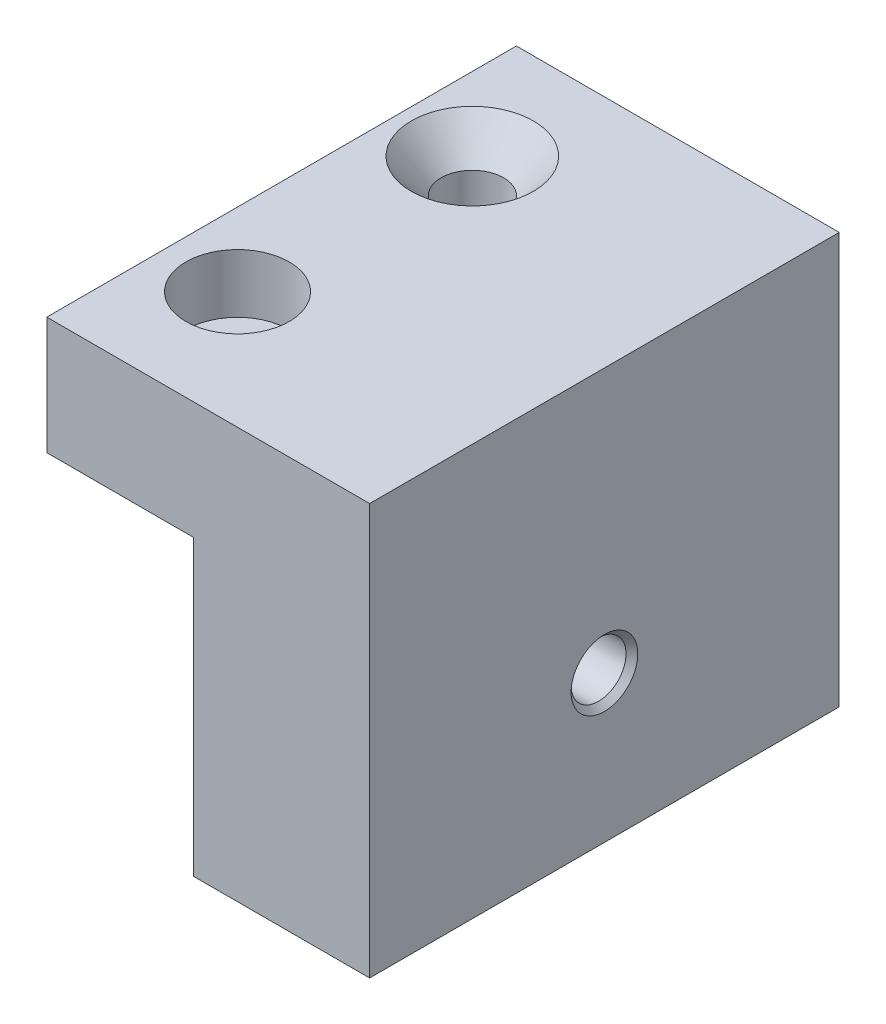
ISO-10303-21;
HEADER;
FILE_DESCRIPTION(('STEP AP214'),'2;1');
FILE_NAME('part.step','',(''),(''),'','','');
FILE_SCHEMA(('AUTOMOTIVE_DESIGN { 1 0 10303 214 1 1 1 1 }'));
ENDSEC;
DATA;
#1=APPLICATION_CONTEXT('core data for automotive mechanical design processes');
#2=APPLICATION_PROTOCOL_DEFINITION('international standard','automotive_design',2000,#1);
#3=PRODUCT_CONTEXT('',#1,'mechanical');
#4=PRODUCT('Part','Part','',(#3));
#5=PRODUCT_RELATED_PRODUCT_CATEGORY('part','',(#4));
#6=PRODUCT_DEFINITION_FORMATION('','',#4);
#7=PRODUCT_DEFINITION_CONTEXT('part definition',#1,'design');
#8=PRODUCT_DEFINITION('design','',#6,#7);
#9=PRODUCT_DEFINITION_SHAPE('','',#8);
#10=(LENGTH_UNIT() NAMED_UNIT(*) SI_UNIT(.MILLI.,.METRE.));
#11=(NAMED_UNIT(*) PLANE_ANGLE_UNIT() SI_UNIT($,.RADIAN.));
#12=(NAMED_UNIT(*) SI_UNIT($,.STERADIAN.) SOLID_ANGLE_UNIT());
#13=UNCERTAINTY_MEASURE_WITH_UNIT(LENGTH_MEASURE(1.E-05),#10,'distance_accuracy_value','');
#14=(GEOMETRIC_REPRESENTATION_CONTEXT(3) GLOBAL_UNCERTAINTY_ASSIGNED_CONTEXT((#13)) GLOBAL_UNIT_ASSIGNED_CONTEXT((#10,
#11,#12)) REPRESENTATION_CONTEXT('',''));
#15=CARTESIAN_POINT('',(0.,0.,0.));
#16=DIRECTION('',(0.,0.,1.));
#17=DIRECTION('',(1.,0.,0.));
#18=AXIS2_PLACEMENT_3D('',#15,#16,#17);
#19=CARTESIAN_POINT('',(-15.875,0.,50.8));
#20=DIRECTION('',(1.,0.,0.));
#21=DIRECTION('',(0.,0.,-1.));
#22=AXIS2_PLACEMENT_3D('',#19,#20,#21);
#23=PLANE('',#22);
#24=DIRECTION('',(0.,-1.,0.));
#25=VECTOR('',#24,1.);
#26=CARTESIAN_POINT('',(-15.875,0.,0.));
#27=LINE('',#26,#25);
#28=CARTESIAN_POINT('',(-15.875,12.7,0.));
#29=VERTEX_POINT('',#28);
#30=CARTESIAN_POINT('',(-15.875,0.,0.));
#31=VERTEX_POINT('',#30);
#32=EDGE_CURVE('E137',#29,#31,#27,.T.);
#33=ORIENTED_EDGE('',*,*,#32,.T.);
#34=DIRECTION('',(0.,0.,-1.));
#35=VECTOR('',#34,1.);
#36=CARTESIAN_POINT('',(-15.875,0.,50.8));
#37=LINE('',#36,#35);
#38=CARTESIAN_POINT('',(-15.875,0.,50.8));
#39=VERTEX_POINT('',#38);
#40=EDGE_CURVE('E146',#39,#31,#37,.T.);
#41=ORIENTED_EDGE('',*,*,#40,.F.);
#42=DIRECTION('',(0.,-1.,0.));
#43=VECTOR('',#42,1.);
#44=CARTESIAN_POINT('',(-15.875,0.,50.8));
#45=LINE('',#44,#43);
#46=CARTESIAN_POINT('',(-15.875,12.7,50.8));
#47=VERTEX_POINT('',#46);
#48=EDGE_CURVE('E103',#47,#39,#45,.T.);
#49=ORIENTED_EDGE('',*,*,#48,.F.);
#50=DIRECTION('',(0.,0.,-1.));
#51=VECTOR('',#50,1.);
#52=CARTESIAN_POINT('',(-15.875,12.7,50.8));
#53=LINE('',#52,#51);
#54=EDGE_CURVE('E155',#47,#29,#53,.T.);
#55=ORIENTED_EDGE('',*,*,#54,.T.);
#56=EDGE_LOOP('',(#33,#41,#49,#55));
#57=FACE_BOUND('',#56,.T.);
#58=ADVANCED_FACE('F41',(#57),#23,.F.);
#59=CARTESIAN_POINT('',(0.,0.,50.8));
#60=DIRECTION('',(0.,1.,0.));
#61=DIRECTION('',(-1.,0.,0.));
#62=AXIS2_PLACEMENT_3D('',#59,#60,#61);
#63=PLANE('',#62);
#64=CARTESIAN_POINT('',(-7.93749999999999,0.,38.1));
#65=DIRECTION('',(0.,1.,0.));
#66=DIRECTION('',(-1.,0.,0.));
#67=AXIS2_PLACEMENT_3D('',#64,#65,#66);
#68=CIRCLE('',#67,3.37819999999999);
#69=CARTESIAN_POINT('',(-11.3157,0.,38.1));
#70=VERTEX_POINT('',#69);
#71=EDGE_CURVE('E46',#70,#70,#68,.T.);
#72=ORIENTED_EDGE('',*,*,#71,.T.);
#73=EDGE_LOOP('',(#72));
#74=FACE_BOUND('',#73,.T.);
#75=CARTESIAN_POINT('',(-7.93749999999999,0.,12.7));
#76=DIRECTION('',(0.,1.,0.));
#77=DIRECTION('',(-1.,0.,0.));
#78=AXIS2_PLACEMENT_3D('',#75,#76,#77);
#79=CIRCLE('',#78,3.3782);
#80=CARTESIAN_POINT('',(-11.3157,0.,12.7));
#81=VERTEX_POINT('',#80);
#82=EDGE_CURVE('E163',#81,#81,#79,.T.);
#83=ORIENTED_EDGE('',*,*,#82,.T.);
#84=EDGE_LOOP('',(#83));
#85=FACE_BOUND('',#84,.T.);
#86=CARTESIAN_POINT('',(-7.9375,0.,25.4));
#87=DIRECTION('',(0.,-1.,0.));
#88=DIRECTION('',(0.,0.,-1.));
#89=AXIS2_PLACEMENT_3D('',#86,#87,#88);
#90=CIRCLE('',#89,1.6002);
#91=CARTESIAN_POINT('',(-7.9375,0.,23.7998));
#92=VERTEX_POINT('',#91);
#93=EDGE_CURVE('E161',#92,#92,#90,.T.);
#94=ORIENTED_EDGE('',*,*,#93,.F.);
#95=EDGE_LOOP('',(#94));
#96=FACE_BOUND('',#95,.T.);
#97=DIRECTION('',(1.,0.,0.));
#98=VECTOR('',#97,1.);
#99=CARTESIAN_POINT('',(0.,0.,0.));
#100=LINE('',#99,#98);
#101=CARTESIAN_POINT('',(0.,0.,0.));
#102=VERTEX_POINT('',#101);
#103=EDGE_CURVE('E139',#31,#102,#100,.T.);
#104=ORIENTED_EDGE('',*,*,#103,.T.);
#105=DIRECTION('',(0.,0.,-1.));
#106=VECTOR('',#105,1.);
#107=CARTESIAN_POINT('',(0.,0.,50.8));
#108=LINE('',#107,#106);
#109=CARTESIAN_POINT('',(0.,0.,50.8));
#110=VERTEX_POINT('',#109);
#111=EDGE_CURVE('E123',#110,#102,#108,.T.);
#112=ORIENTED_EDGE('',*,*,#111,.F.);
#113=DIRECTION('',(1.,0.,0.));
#114=VECTOR('',#113,1.);
#115=CARTESIAN_POINT('',(0.,0.,50.8));
#116=LINE('',#115,#114);
#117=EDGE_CURVE('E116',#39,#110,#116,.T.);
#118=ORIENTED_EDGE('',*,*,#117,.F.);
#119=ORIENTED_EDGE('',*,*,#40,.T.);
#120=EDGE_LOOP('',(#104,#112,#118,#119));
#121=FACE_BOUND('',#120,.T.);
#122=ADVANCED_FACE('F183',(#74,#85,#96,#121),#63,.F.);
#123=CARTESIAN_POINT('',(0.,0.,50.8));
#124=DIRECTION('',(1.,0.,0.));
#125=DIRECTION('',(0.,1.,0.));
#126=AXIS2_PLACEMENT_3D('',#123,#124,#125);
#127=PLANE('',#126);
#128=CARTESIAN_POINT('',(0.,-15.875,25.4));
#129=DIRECTION('',(1.,0.,0.));
#130=DIRECTION('',(0.,1.,0.));
#131=AXIS2_PLACEMENT_3D('',#128,#129,#130);
#132=CIRCLE('',#131,3.6068);
#133=CARTESIAN_POINT('',(0.,-12.2682,25.4));
#134=VERTEX_POINT('',#133);
#135=EDGE_CURVE('E11',#134,#134,#132,.T.);
#136=ORIENTED_EDGE('',*,*,#135,.T.);
#137=EDGE_LOOP('',(#136));
#138=FACE_BOUND('',#137,.T.);
#139=DIRECTION('',(0.,-1.,0.));
#140=VECTOR('',#139,1.);
#141=CARTESIAN_POINT('',(0.,0.,0.));
#142=LINE('',#141,#140);
#143=CARTESIAN_POINT('',(0.,-31.75,0.));
#144=VERTEX_POINT('',#143);
#145=EDGE_CURVE('E121',#102,#144,#142,.T.);
#146=ORIENTED_EDGE('',*,*,#145,.T.);
#147=DIRECTION('',(0.,0.,-1.));
#148=VECTOR('',#147,1.);
#149=CARTESIAN_POINT('',(0.,-31.75,50.8));
#150=LINE('',#149,#148);
#151=CARTESIAN_POINT('',(0.,-31.75,50.8));
#152=VERTEX_POINT('',#151);
#153=EDGE_CURVE('E122',#152,#144,#150,.T.);
#154=ORIENTED_EDGE('',*,*,#153,.F.);
#155=DIRECTION('',(0.,-1.,0.));
#156=VECTOR('',#155,1.);
#157=CARTESIAN_POINT('',(0.,0.,50.8));
#158=LINE('',#157,#156);
#159=EDGE_CURVE('E109',#110,#152,#158,.T.);
#160=ORIENTED_EDGE('',*,*,#159,.F.);
#161=ORIENTED_EDGE('',*,*,#111,.T.);
#162=EDGE_LOOP('',(#146,#154,#160,#161));
#163=FACE_BOUND('',#162,.T.);
#164=ADVANCED_FACE('F125',(#138,#163),#127,.F.);
#165=CARTESIAN_POINT('',(0.,-31.75,50.8));
#166=DIRECTION('',(0.,1.,0.));
#167=DIRECTION('',(0.,0.,1.));
#168=AXIS2_PLACEMENT_3D('',#165,#166,#167);
#169=PLANE('',#168);
#170=DIRECTION('',(1.,0.,0.));
#171=VECTOR('',#170,1.);
#172=CARTESIAN_POINT('',(0.,-31.75,0.));
#173=LINE('',#172,#171);
#174=CARTESIAN_POINT('',(19.05,-31.75,0.));
#175=VERTEX_POINT('',#174);
#176=EDGE_CURVE('E86',#144,#175,#173,.T.);
#177=ORIENTED_EDGE('',*,*,#176,.T.);
#178=DIRECTION('',(0.,0.,-1.));
#179=VECTOR('',#178,1.);
#180=CARTESIAN_POINT('',(19.05,-31.75,50.8));
#181=LINE('',#180,#179);
#182=CARTESIAN_POINT('',(19.05,-31.75,50.8));
#183=VERTEX_POINT('',#182);
#184=EDGE_CURVE('E127',#183,#175,#181,.T.);
#185=ORIENTED_EDGE('',*,*,#184,.F.);
#186=DIRECTION('',(1.,0.,0.));
#187=VECTOR('',#186,1.);
#188=CARTESIAN_POINT('',(0.,-31.75,50.8));
#189=LINE('',#188,#187);
#190=EDGE_CURVE('E112',#152,#183,#189,.T.);
#191=ORIENTED_EDGE('',*,*,#190,.F.);
#192=ORIENTED_EDGE('',*,*,#153,.T.);
#193=EDGE_LOOP('',(#177,#185,#191,#192));
#194=FACE_BOUND('',#193,.T.);
#195=ADVANCED_FACE('F129',(#194),#169,.F.);
#196=CARTESIAN_POINT('',(19.05,12.7,50.8));
#197=DIRECTION('',(-1.,0.,0.));
#198=DIRECTION('',(0.,-1.,0.));
#199=AXIS2_PLACEMENT_3D('',#196,#197,#198);
#200=PLANE('',#199);
#201=CARTESIAN_POINT('',(19.05,-15.875,25.4));
#202=DIRECTION('',(-1.,0.,0.));
#203=DIRECTION('',(0.,-1.,0.));
#204=AXIS2_PLACEMENT_3D('',#201,#202,#203);
#205=CIRCLE('',#204,3.6068);
#206=CARTESIAN_POINT('',(19.05,-19.4818,25.4));
#207=VERTEX_POINT('',#206);
#208=EDGE_CURVE('E153',#207,#207,#205,.T.);
#209=ORIENTED_EDGE('',*,*,#208,.T.);
#210=EDGE_LOOP('',(#209));
#211=FACE_BOUND('',#210,.T.);
#212=DIRECTION('',(0.,1.,0.));
#213=VECTOR('',#212,1.);
#214=CARTESIAN_POINT('',(19.05,12.7,0.));
#215=LINE('',#214,#213);
#216=CARTESIAN_POINT('',(19.05,12.7,0.));
#217=VERTEX_POINT('',#216);
#218=EDGE_CURVE('E94',#175,#217,#215,.T.);
#219=ORIENTED_EDGE('',*,*,#218,.T.);
#220=DIRECTION('',(0.,0.,-1.));
#221=VECTOR('',#220,1.);
#222=CARTESIAN_POINT('',(19.05,12.7,50.8));
#223=LINE('',#222,#221);
#224=CARTESIAN_POINT('',(19.05,12.7,50.8));
#225=VERTEX_POINT('',#224);
#226=EDGE_CURVE('E135',#225,#217,#223,.T.);
#227=ORIENTED_EDGE('',*,*,#226,.F.);
#228=DIRECTION('',(0.,1.,0.));
#229=VECTOR('',#228,1.);
#230=CARTESIAN_POINT('',(19.05,12.7,50.8));
#231=LINE('',#230,#229);
#232=EDGE_CURVE('E128',#183,#225,#231,.T.);
#233=ORIENTED_EDGE('',*,*,#232,.F.);
#234=ORIENTED_EDGE('',*,*,#184,.T.);
#235=EDGE_LOOP('',(#219,#227,#233,#234));
#236=FACE_BOUND('',#235,.T.);
#237=ADVANCED_FACE('F186',(#211,#236),#200,.F.);
#238=CARTESIAN_POINT('',(0.,12.7,50.8));
#239=DIRECTION('',(0.,-1.,0.));
#240=DIRECTION('',(0.,0.,-1.));
#241=AXIS2_PLACEMENT_3D('',#238,#239,#240);
#242=PLANE('',#241);
#243=CARTESIAN_POINT('',(-7.93749999999999,12.7,38.1));
#244=DIRECTION('',(0.,1.,0.));
#245=DIRECTION('',(0.,0.,1.));
#246=AXIS2_PLACEMENT_3D('',#243,#244,#245);
#247=CIRCLE('',#246,5.588);
#248=CARTESIAN_POINT('',(-7.93749999999999,12.7,43.688));
#249=VERTEX_POINT('',#248);
#250=EDGE_CURVE('E380',#249,#249,#247,.T.);
#251=ORIENTED_EDGE('',*,*,#250,.F.);
#252=EDGE_LOOP('',(#251));
#253=FACE_BOUND('',#252,.T.);
#254=CARTESIAN_POINT('',(-7.93749999999999,12.7,12.7));
#255=DIRECTION('',(0.,1.,0.));
#256=DIRECTION('',(0.,0.,1.));
#257=AXIS2_PLACEMENT_3D('',#254,#255,#256);
#258=CIRCLE('',#257,6.604);
#259=CARTESIAN_POINT('',(-7.93749999999999,12.7,19.304));
#260=VERTEX_POINT('',#259);
#261=EDGE_CURVE('E167',#260,#260,#258,.T.);
#262=ORIENTED_EDGE('',*,*,#261,.F.);
#263=EDGE_LOOP('',(#262));
#264=FACE_BOUND('',#263,.T.);
#265=DIRECTION('',(-1.,0.,0.));
#266=VECTOR('',#265,1.);
#267=CARTESIAN_POINT('',(0.,12.7,0.));
#268=LINE('',#267,#266);
#269=EDGE_CURVE('E144',#217,#29,#268,.T.);
#270=ORIENTED_EDGE('',*,*,#269,.T.);
#271=ORIENTED_EDGE('',*,*,#54,.F.);
#272=DIRECTION('',(-1.,0.,0.));
#273=VECTOR('',#272,1.);
#274=CARTESIAN_POINT('',(0.,12.7,50.8));
#275=LINE('',#274,#273);
#276=EDGE_CURVE('E62',#225,#47,#275,.T.);
#277=ORIENTED_EDGE('',*,*,#276,.F.);
#278=ORIENTED_EDGE('',*,*,#226,.T.);
#279=EDGE_LOOP('',(#270,#271,#277,#278));
#280=FACE_BOUND('',#279,.T.);
#281=ADVANCED_FACE('F189',(#253,#264,#280),#242,.F.);
#282=CARTESIAN_POINT('',(0.,0.,50.8));
#283=DIRECTION('',(0.,0.,-1.));
#284=DIRECTION('',(-1.,0.,0.));
#285=AXIS2_PLACEMENT_3D('',#282,#283,#284);
#286=PLANE('',#285);
#287=ORIENTED_EDGE('',*,*,#276,.T.);
#288=ORIENTED_EDGE('',*,*,#48,.T.);
#289=ORIENTED_EDGE('',*,*,#117,.T.);
#290=ORIENTED_EDGE('',*,*,#159,.T.);
#291=ORIENTED_EDGE('',*,*,#190,.T.);
#292=ORIENTED_EDGE('',*,*,#232,.T.);
#293=EDGE_LOOP('',(#287,#288,#289,#290,#291,#292));
#294=FACE_BOUND('',#293,.T.);
#295=ADVANCED_FACE('F115',(#294),#286,.F.);
#296=CARTESIAN_POINT('',(0.,0.,0.));
#297=DIRECTION('',(0.,0.,-1.));
#298=DIRECTION('',(-1.,0.,0.));
#299=AXIS2_PLACEMENT_3D('',#296,#297,#298);
#300=PLANE('',#299);
#301=ORIENTED_EDGE('',*,*,#32,.F.);
#302=ORIENTED_EDGE('',*,*,#269,.F.);
#303=ORIENTED_EDGE('',*,*,#218,.F.);
#304=ORIENTED_EDGE('',*,*,#176,.F.);
#305=ORIENTED_EDGE('',*,*,#145,.F.);
#306=ORIENTED_EDGE('',*,*,#103,.F.);
#307=EDGE_LOOP('',(#301,#302,#303,#304,#305,#306));
#308=FACE_BOUND('',#307,.T.);
#309=ADVANCED_FACE('F187',(#308),#300,.T.);
#310=CARTESIAN_POINT('',(0.,-15.875,25.4));
#311=DIRECTION('',(-1.,0.,0.));
#312=DIRECTION('',(0.,0.,1.));
#313=AXIS2_PLACEMENT_3D('',#310,#311,#312);
#314=CYLINDRICAL_SURFACE('',#313,2.97179999999999);
#315=CARTESIAN_POINT('',(18.415,-15.875,25.4));
#316=DIRECTION('',(-1.,0.,0.));
#317=DIRECTION('',(0.,0.,1.));
#318=AXIS2_PLACEMENT_3D('',#315,#316,#317);
#319=CIRCLE('',#318,2.97179999999999);
#320=CARTESIAN_POINT('',(18.415,-15.875,28.3718));
#321=VERTEX_POINT('',#320);
#322=EDGE_CURVE('E55',#321,#321,#319,.F.);
#323=ORIENTED_EDGE('',*,*,#322,.T.);
#324=EDGE_LOOP('',(#323));
#325=FACE_BOUND('',#324,.T.);
#326=CARTESIAN_POINT('',(0.635,-15.875,25.4));
#327=DIRECTION('',(1.,0.,0.));
#328=DIRECTION('',(0.,0.,-1.));
#329=AXIS2_PLACEMENT_3D('',#326,#327,#328);
#330=CIRCLE('',#329,2.97179999999999);
#331=CARTESIAN_POINT('',(0.635,-15.875,22.4282));
#332=VERTEX_POINT('',#331);
#333=EDGE_CURVE('E160',#332,#332,#330,.F.);
#334=ORIENTED_EDGE('',*,*,#333,.T.);
#335=EDGE_LOOP('',(#334));
#336=FACE_BOUND('',#335,.T.);
#337=ADVANCED_FACE('F213',(#325,#336),#314,.F.);
#338=CARTESIAN_POINT('',(19.05,-15.875,25.4));
#339=DIRECTION('',(1.,0.,0.));
#340=DIRECTION('',(0.,0.,-1.));
#341=AXIS2_PLACEMENT_3D('',#338,#339,#340);
#342=CONICAL_SURFACE('',#341,3.6068,0.785398163397441);
#343=ORIENTED_EDGE('',*,*,#322,.F.);
#344=EDGE_LOOP('',(#343));
#345=FACE_BOUND('',#344,.T.);
#346=ORIENTED_EDGE('',*,*,#208,.F.);
#347=EDGE_LOOP('',(#346));
#348=FACE_BOUND('',#347,.T.);
#349=ADVANCED_FACE('F212',(#345,#348),#342,.F.);
#350=CARTESIAN_POINT('',(0.635,-15.875,25.4));
#351=DIRECTION('',(-1.,0.,0.));
#352=DIRECTION('',(0.,0.,1.));
#353=AXIS2_PLACEMENT_3D('',#350,#351,#352);
#354=CONICAL_SURFACE('',#353,2.97179999999999,0.785398163397453);
#355=ORIENTED_EDGE('',*,*,#135,.F.);
#356=EDGE_LOOP('',(#355));
#357=FACE_BOUND('',#356,.T.);
#358=ORIENTED_EDGE('',*,*,#333,.F.);
#359=EDGE_LOOP('',(#358));
#360=FACE_BOUND('',#359,.T.);
#361=ADVANCED_FACE('F42',(#357,#360),#354,.F.);
#362=CARTESIAN_POINT('',(-7.9375,6.0198,25.4));
#363=DIRECTION('',(0.,-1.,0.));
#364=DIRECTION('',(0.,0.,-1.));
#365=AXIS2_PLACEMENT_3D('',#362,#363,#364);
#366=CONICAL_SURFACE('',#365,1.6002,0.785398163397447);
#367=CARTESIAN_POINT('',(-7.9375,7.62,25.4));
#368=VERTEX_POINT('',#367);
#369=VERTEX_LOOP('',#368);
#370=FACE_BOUND('',#369,.T.);
#371=CARTESIAN_POINT('',(-7.9375,6.0198,25.4));
#372=DIRECTION('',(0.,-1.,0.));
#373=DIRECTION('',(0.,0.,-1.));
#374=AXIS2_PLACEMENT_3D('',#371,#372,#373);
#375=CIRCLE('',#374,1.6002);
#376=CARTESIAN_POINT('',(-7.9375,6.0198,23.7998));
#377=VERTEX_POINT('',#376);
#378=EDGE_CURVE('E136',#377,#377,#375,.T.);
#379=ORIENTED_EDGE('',*,*,#378,.T.);
#380=EDGE_LOOP('',(#379));
#381=FACE_BOUND('',#380,.T.);
#382=ADVANCED_FACE('F219',(#370,#381),#366,.F.);
#383=CARTESIAN_POINT('',(-7.9375,0.,25.4));
#384=DIRECTION('',(0.,-1.,0.));
#385=DIRECTION('',(0.,0.,-1.));
#386=AXIS2_PLACEMENT_3D('',#383,#384,#385);
#387=CYLINDRICAL_SURFACE('',#386,1.6002);
#388=ORIENTED_EDGE('',*,*,#378,.F.);
#389=EDGE_LOOP('',(#388));
#390=FACE_BOUND('',#389,.T.);
#391=ORIENTED_EDGE('',*,*,#93,.T.);
#392=EDGE_LOOP('',(#391));
#393=FACE_BOUND('',#392,.T.);
#394=ADVANCED_FACE('F321',(#390,#393),#387,.F.);
#395=CARTESIAN_POINT('',(-7.93749999999999,12.7,12.7));
#396=DIRECTION('',(0.,1.,0.));
#397=DIRECTION('',(0.,0.,1.));
#398=AXIS2_PLACEMENT_3D('',#395,#396,#397);
#399=CYLINDRICAL_SURFACE('',#398,3.3782);
#400=CARTESIAN_POINT('',(-7.93749999999999,8.98914159198646,12.7));
#401=DIRECTION('',(0.,1.,0.));
#402=DIRECTION('',(0.,0.,1.));
#403=AXIS2_PLACEMENT_3D('',#400,#401,#402);
#404=CIRCLE('',#403,3.3782);
#405=CARTESIAN_POINT('',(-7.93749999999999,8.98914159198646,16.0782));
#406=VERTEX_POINT('',#405);
#407=EDGE_CURVE('E165',#406,#406,#404,.T.);
#408=ORIENTED_EDGE('',*,*,#407,.T.);
#409=EDGE_LOOP('',(#408));
#410=FACE_BOUND('',#409,.T.);
#411=ORIENTED_EDGE('',*,*,#82,.F.);
#412=EDGE_LOOP('',(#411));
#413=FACE_BOUND('',#412,.T.);
#414=ADVANCED_FACE('F314',(#410,#413),#399,.F.);
#415=CARTESIAN_POINT('',(-7.93749999999999,12.7,12.7));
#416=DIRECTION('',(0.,1.,0.));
#417=DIRECTION('',(0.,0.,1.));
#418=AXIS2_PLACEMENT_3D('',#415,#416,#417);
#419=CONICAL_SURFACE('',#418,6.604,0.715584993317675);
#420=ORIENTED_EDGE('',*,*,#407,.F.);
#421=EDGE_LOOP('',(#420));
#422=FACE_BOUND('',#421,.T.);
#423=ORIENTED_EDGE('',*,*,#261,.T.);
#424=EDGE_LOOP('',(#423));
#425=FACE_BOUND('',#424,.T.);
#426=ADVANCED_FACE('F287',(#422,#425),#419,.F.);
#427=CARTESIAN_POINT('',(-7.93749999999999,12.7,38.1));
#428=DIRECTION('',(0.,1.,0.));
#429=DIRECTION('',(0.,0.,1.));
#430=AXIS2_PLACEMENT_3D('',#427,#428,#429);
#431=CYLINDRICAL_SURFACE('',#430,3.37819999999999);
#432=CARTESIAN_POINT('',(-7.93749999999999,6.35,38.1));
#433=DIRECTION('',(0.,1.,0.));
#434=DIRECTION('',(0.,0.,1.));
#435=AXIS2_PLACEMENT_3D('',#432,#433,#434);
#436=CIRCLE('',#435,3.3782);
#437=CARTESIAN_POINT('',(-7.93749999999999,6.35,41.4782));
#438=VERTEX_POINT('',#437);
#439=EDGE_CURVE('E378',#438,#438,#436,.T.);
#440=ORIENTED_EDGE('',*,*,#439,.T.);
#441=EDGE_LOOP('',(#440));
#442=FACE_BOUND('',#441,.T.);
#443=ORIENTED_EDGE('',*,*,#71,.F.);
#444=EDGE_LOOP('',(#443));
#445=FACE_BOUND('',#444,.T.);
#446=ADVANCED_FACE('F281',(#442,#445),#431,.F.);
#447=CARTESIAN_POINT('',(-4.55929999999999,6.35,38.1));
#448=DIRECTION('',(0.,-1.,0.));
#449=DIRECTION('',(0.,0.,-1.));
#450=AXIS2_PLACEMENT_3D('',#447,#448,#449);
#451=PLANE('',#450);
#452=ORIENTED_EDGE('',*,*,#439,.F.);
#453=EDGE_LOOP('',(#452));
#454=FACE_BOUND('',#453,.T.);
#455=CARTESIAN_POINT('',(-7.93749999999999,6.35,38.1));
#456=DIRECTION('',(0.,1.,0.));
#457=DIRECTION('',(0.,0.,1.));
#458=AXIS2_PLACEMENT_3D('',#455,#456,#457);
#459=CIRCLE('',#458,5.588);
#460=CARTESIAN_POINT('',(-7.93749999999999,6.35,43.688));
#461=VERTEX_POINT('',#460);
#462=EDGE_CURVE('E372',#461,#461,#459,.T.);
#463=ORIENTED_EDGE('',*,*,#462,.T.);
#464=EDGE_LOOP('',(#463));
#465=FACE_BOUND('',#464,.T.);
#466=ADVANCED_FACE('F284',(#454,#465),#451,.F.);
#467=CARTESIAN_POINT('',(-7.93749999999999,12.7,38.1));
#468=DIRECTION('',(0.,1.,0.));
#469=DIRECTION('',(0.,0.,1.));
#470=AXIS2_PLACEMENT_3D('',#467,#468,#469);
#471=CYLINDRICAL_SURFACE('',#470,5.588);
#472=ORIENTED_EDGE('',*,*,#462,.F.);
#473=EDGE_LOOP('',(#472));
#474=FACE_BOUND('',#473,.T.);
#475=ORIENTED_EDGE('',*,*,#250,.T.);
#476=EDGE_LOOP('',(#475));
#477=FACE_BOUND('',#476,.T.);
#478=ADVANCED_FACE('F298',(#474,#477),#471,.F.);
#479=CLOSED_SHELL('',(#58,#122,#164,#195,#237,#281,#295,#309,#337,#349,#361,#382,#394,#414,#426,
#446,#466,#478));
#480=MANIFOLD_SOLID_BREP('B2',#479);
#481=ADVANCED_BREP_SHAPE_REPRESENTATION('',(#18,#480),#14);
#482=SHAPE_DEFINITION_REPRESENTATION(#9,#481);
ENDSEC;
END-ISO-10303-21;
